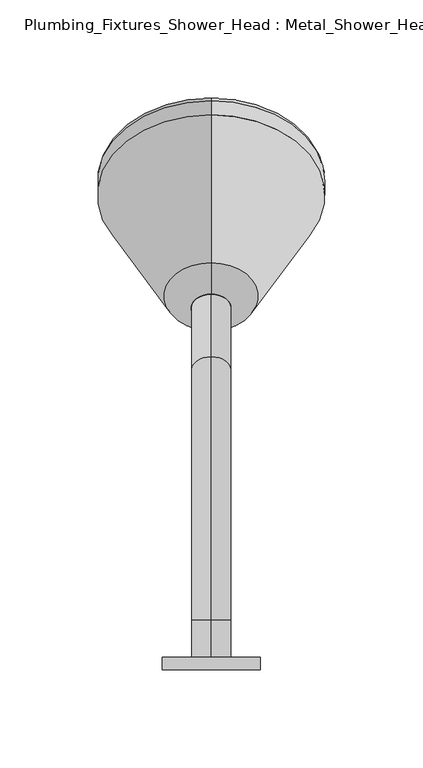
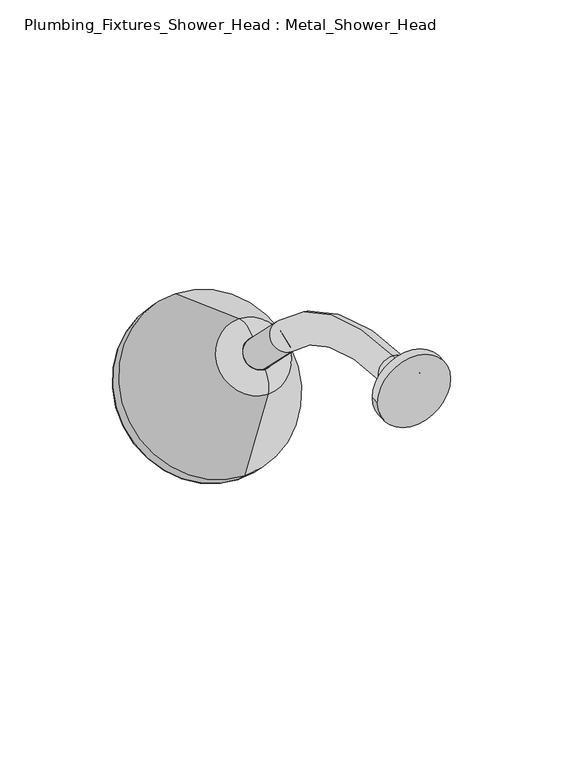
"""IFC4 building model written with IfcOpenShell, lengths in millimetres: flow terminal geometry, Plumbing_Fixtures_Shower_Head : Metal_Shower_Head."""

from ifc_helpers import new_model, si_unit, point, frame, frame_2d, origin, place, context, project, spatial, polyline, circle_curve, ellipse_curve, trimmed, segment, composite_curve, outline, extrude, source, transform, mapped, element, save
from ifc_brep_helpers import plane_surface, cylinder_surface, revolved_surface, advanced_brep


def plumbing_fixtures_shower_head_metal_shower_head_9404fff0(model_context):
    return source(origin(), model_context, "Body", "SolidModel", [
        advanced_brep(
        [(0.0, 6.4821489, 1590.0), (0.0, 6.4821489, 1610.0), (0.0, 25.4415588, 1590.0), (0.0, 25.4415588, 1610.0), (0.0, 159.7918472, 1554.3502884), (0.0, 145.6497116, 1540.2081528), (0.0, 177.4695167, 1508.3883476), (0.0, 191.6116524, 1522.5304833)],
        [
            (0, 1, circle_curve(frame((0.0, 6.4821489, 1600.0), z_axis=(0.0, -1.0, 0.0), x_axis=(0.0, 0.0, 1.0)), 10.0)),
            (1, 0, circle_curve(frame((0.0, 6.4821489, 1600.0), z_axis=(0.0, -1.0, 0.0), x_axis=(0.0, 0.0, 1.0)), 10.0)),
            (0, 2),
            (2, 3, circle_curve(frame((0.0, 25.4415588, 1600.0), z_axis=(0.0, -1.0, 0.0), x_axis=(0.0, 0.0, 1.0)), 10.0)),
            (3, 1),
            (3, 2, circle_curve(frame((0.0, 25.4415588, 1600.0), z_axis=(0.0, -1.0, 0.0), x_axis=(0.0, 0.0, 1.0)), 10.0)),
            (4, 3, circle_curve(frame((0.0, 25.4415588, 1420.0), z_axis=(1.0, 0.0, 0.0), x_axis=(0.0, 0.0, 1.0)), 190.0)),
            (2, 5, circle_curve(frame((0.0, 25.4415588, 1420.0), z_axis=(-1.0, 0.0, 0.0), x_axis=(0.0, 0.0, 1.0)), 170.0)),
            (5, 4, circle_curve(frame((0.0, 152.7207794, 1547.2792206), z_axis=(0.0, -0.7071067811865417, 0.7071067811865533), x_axis=(0.0, 0.7071067811865533, 0.7071067811865417)), 10.0)),
            (4, 5, circle_curve(frame((0.0, 152.7207794, 1547.2792206), z_axis=(0.0, -0.7071067811865416, 0.7071067811865535), x_axis=(0.0, 0.7071067811865535, 0.7071067811865416)), 10.0)),
            (6, 7, circle_curve(frame((0.0, 184.5405845, 1515.4594155), z_axis=(0.0, 0.7071067811865412, -0.7071067811865539), x_axis=(0.0, 0.7071067811865539, 0.7071067811865412)), 10.0)),
            (7, 6, circle_curve(frame((0.0, 184.5405845, 1515.4594155), z_axis=(0.0, 0.7071067811865412, -0.7071067811865539), x_axis=(0.0, 0.7071067811865539, 0.7071067811865412)), 10.0)),
            (5, 6),
            (7, 4),
        ],
        [
            plane_surface(frame((0.0, 6.4821489, 1600.0), z_axis=(0.0, -1.0, 0.0), x_axis=(1.0, 0.0, 0.0))),
            cylinder_surface(frame((0.0, 6.4821489, 1600.0), z_axis=(0.0, -1.0, 0.0), x_axis=(0.0, 0.0, 1.0)), 10.0),
            revolved_surface(trimmed(ellipse_curve(frame((0.0, 25.4415588, 1600.0), z_axis=(0.0, -1.0, 0.0), x_axis=(0.0, 0.0, 1.0)), 10.0, 10.0), [point((0.0, 25.4415588, 1590.0))], [point((0.0, 25.4415588, 1610.0))], True, "CARTESIAN"), (0.0, 25.4415588, 1420.0), (-1.0, 0.0, 0.0)),
            revolved_surface(trimmed(ellipse_curve(frame((0.0, 25.4415588, 1600.0), z_axis=(0.0, -1.0, 0.0), x_axis=(0.0, 0.0, 1.0)), 10.0, 10.0), [point((0.0, 25.4415588, 1610.0))], [point((0.0, 25.4415588, 1590.0))], True, "CARTESIAN"), (0.0, 25.4415588, 1420.0), (-1.0, 0.0, 0.0)),
            plane_surface(frame((0.0, 184.5405845, 1515.4594155), z_axis=(0.0, 0.7071067811865412, -0.7071067811865539), x_axis=(1.0, 0.0, 0.0))),
            cylinder_surface(frame((0.0, 152.7207794, 1547.2792206), z_axis=(0.0, -0.7071067811865412, 0.7071067811865539), x_axis=(0.0, 0.7071067811865539, 0.7071067811865412)), 10.0),
        ],
        [
            (0, [[1, 2]]),
            (1, [[-1, 3, 4, 5]]),
            (1, [[-2, -5, 6, -3]]),
            (2, [[7, -4, 8, 9]]),
            (3, [[-8, -6, -7, 10]]),
            (4, [[11, 12]]),
            (5, [[-9, 13, -12, 14]]),
            (5, [[-10, -14, -11, -13]]),
        ],
    ),
        advanced_brep(
        [(0.0, 207.6624735, 1526.3331882), (0.0, 173.6668118, 1492.3375265), (0.0, 177.1555994, 1508.0744304), (0.0, 191.9255696, 1522.8444006), (0.0, 283.255056, 1498.8197382), (0.0, 201.1802618, 1416.744944), (0.0, 290.3261238, 1491.7486704), (0.0, 208.2513296, 1409.6738762), (0.0, 290.3261238, 1484.6776026), (0.0, 215.3223974, 1409.6738762), (0.0, 288.6229509, 1482.9744296), (0.0, 217.0255704, 1411.3770491), (0.0, 287.2087373, 1484.3886432), (0.0, 215.6113568, 1412.7912627), (0.0, 251.4100471, 1448.5899529), (0.0, 184.5405845, 1515.4594155)],
        [
            (0, 1, circle_curve(frame((0.0, 190.6646427, 1509.3353573), z_axis=(0.0, -0.7071067811865374, 0.7071067811865579), x_axis=(0.0, -0.7071067811865579, -0.7071067811865374)), 24.0385629)),
            (1, 2, circle_curve(frame((0.0, 187.7622012, 1497.4678286), z_axis=(-1.0000000000000002, 0.0, 0.0), x_axis=(0.0, 1.0000000000000002, 0.0)), 15.0)),
            (2, 3, circle_curve(frame((0.0, 184.5405845, 1515.4594155), z_axis=(0.0, 0.7071067811865374, -0.7071067811865579), x_axis=(0.0, -0.7071067811865579, -0.7071067811865374)), 10.4439461)),
            (3, 0, circle_curve(frame((0.0, 202.5321714, 1512.2377988), z_axis=(-1.0000000000000002, 0.0, 0.0), x_axis=(0.0, 0.0, -1.0000000000000002)), 15.0)),
            (1, 0, circle_curve(frame((0.0, 190.6646427, 1509.3353573), z_axis=(0.0, -0.7071067811865374, 0.7071067811865579), x_axis=(0.0, -0.7071067811865579, -0.7071067811865374)), 24.0385629)),
            (3, 2, circle_curve(frame((0.0, 184.5405845, 1515.4594155), z_axis=(0.0, 0.7071067811865374, -0.7071067811865579), x_axis=(0.0, -0.7071067811865579, -0.7071067811865374)), 10.4439461)),
            (4, 5, circle_curve(frame((0.0, 242.2176589, 1457.7823411), z_axis=(0.0, -0.7071067811865374, 0.7071067811865579), x_axis=(0.0, -0.7071067811865579, -0.7071067811865374)), 58.0356436)),
            (5, 1),
            (0, 4),
            (5, 4, circle_curve(frame((0.0, 242.2176589, 1457.7823411), z_axis=(0.0, -0.7071067811865374, 0.7071067811865579), x_axis=(0.0, -0.7071067811865579, -0.7071067811865374)), 58.0356436)),
            (6, 7, circle_curve(frame((0.0, 249.2887267, 1450.7112733), z_axis=(0.0, -0.7071067811865374, 0.7071067811865579), x_axis=(0.0, -0.7071067811865579, -0.7071067811865374)), 58.0356436)),
            (7, 5),
            (4, 6),
            (7, 6, circle_curve(frame((0.0, 249.2887267, 1450.7112733), z_axis=(0.0, -0.7071067811865374, 0.7071067811865579), x_axis=(0.0, -0.7071067811865579, -0.7071067811865374)), 58.0356436)),
            (8, 9, circle_curve(frame((0.0, 252.8242606, 1447.1757394), z_axis=(0.0, -0.7071067811865374, 0.7071067811865579), x_axis=(0.0, -0.7071067811865579, -0.7071067811865374)), 53.0356436)),
            (9, 7, circle_curve(frame((0.0, 211.7868635, 1413.2094101), z_axis=(-1.0000000000000002, 0.0, 0.0), x_axis=(0.0, 1.0000000000000002, 0.0)), 5.0)),
            (6, 8, circle_curve(frame((0.0, 286.7905899, 1488.2131365), z_axis=(-1.0000000000000002, 0.0, 0.0), x_axis=(0.0, 0.0, -1.0000000000000002)), 5.0)),
            (9, 8, circle_curve(frame((0.0, 252.8242606, 1447.1757394), z_axis=(0.0, -0.7071067811865374, 0.7071067811865579), x_axis=(0.0, -0.7071067811865579, -0.7071067811865374)), 53.0356436)),
            (10, 11, circle_curve(frame((0.0, 252.8242606, 1447.1757394), z_axis=(0.0, -0.7071067811865374, 0.7071067811865579), x_axis=(0.0, -0.7071067811865579, -0.7071067811865374)), 50.6269933)),
            (11, 9),
            (8, 10),
            (11, 10, circle_curve(frame((0.0, 252.8242606, 1447.1757394), z_axis=(0.0, -0.7071067811865374, 0.7071067811865579), x_axis=(0.0, -0.7071067811865579, -0.7071067811865374)), 50.6269933)),
            (12, 13, circle_curve(frame((0.0, 251.4100471, 1448.5899529), z_axis=(0.0, -0.7071067811865374, 0.7071067811865579), x_axis=(0.0, -0.7071067811865579, -0.7071067811865374)), 50.6269933)),
            (13, 11),
            (10, 12),
            (13, 12, circle_curve(frame((0.0, 251.4100471, 1448.5899529), z_axis=(0.0, -0.7071067811865374, 0.7071067811865579), x_axis=(0.0, -0.7071067811865579, -0.7071067811865374)), 50.6269933)),
            (14, 13),
            (12, 14),
            (2, 15),
            (15, 3),
        ],
        [
            revolved_surface(trimmed(ellipse_curve(frame((0.0, 187.7622012, 1497.4678286), z_axis=(1.0000000000000002, 0.0, 0.0), x_axis=(0.0, 1.0000000000000002, 0.0)), 15.0, 15.0), [point((0.0, 177.1555994, 1508.0744304))], [point((0.0, 173.6668118, 1492.3375265))], True, "CARTESIAN"), (0.0, 184.5405845, 1515.4594155), (0.0, 0.7071067811865374, -0.7071067811865579)),
            revolved_surface(polyline([(0.0, 173.6668118, 1492.3375265), (0.0, 201.1802618, 1416.744944)]), (0.0, 184.5405845, 1515.4594155), (0.0, 0.7071067811865374, -0.7071067811865579)),
            cylinder_surface(frame((0.0, 184.5405845, 1515.4594155), z_axis=(0.0, 0.7071067811865374, -0.7071067811865579), x_axis=(0.0, -0.7071067811865579, -0.7071067811865374)), 58.0356436),
            revolved_surface(trimmed(ellipse_curve(frame((0.0, 211.7868635, 1413.2094101), z_axis=(1.0000000000000002, 0.0, 0.0), x_axis=(0.0, 1.0000000000000002, 0.0)), 5.0, 5.0), [point((0.0, 208.2513296, 1409.6738762))], [point((0.0, 215.3223974, 1409.6738762))], True, "CARTESIAN"), (0.0, 184.5405845, 1515.4594155), (0.0, 0.7071067811865374, -0.7071067811865579)),
            plane_surface(frame((0.0, 252.8242606, 1447.1757394), z_axis=(0.0, 0.7071067811865374, -0.7071067811865579), x_axis=(0.0, -0.7071067811865579, -0.7071067811865374))),
            revolved_surface(polyline([(0.0, 217.02557037648307, 1411.3770490764832), (0.0, 215.61135677648213, 1412.7912626764842)]), (0.0, 184.5405845, 1515.4594155), (0.0, 0.7071067811865374, -0.7071067811865579)),
            plane_surface(frame((0.0, 251.4100471, 1448.5899529), z_axis=(0.0, 0.7071067811865374, -0.7071067811865579), x_axis=(0.0, -0.7071067811865579, -0.7071067811865374))),
            plane_surface(frame((0.0, 184.5405845, 1515.4594155), z_axis=(0.0, -0.7071067811865374, 0.7071067811865579), x_axis=(0.0, -0.7071067811865579, -0.7071067811865374))),
        ],
        [
            (0, [[1, 2, 3, 4]]),
            (0, [[5, -4, 6, -2]]),
            (1, [[7, 8, -1, 9]]),
            (1, [[10, -9, -5, -8]]),
            (2, [[11, 12, -7, 13]]),
            (2, [[14, -13, -10, -12]]),
            (3, [[15, 16, -11, 17]]),
            (3, [[18, -17, -14, -16]]),
            (4, [[19, 20, -15, 21]]),
            (4, [[22, -21, -18, -20]]),
            (5, [[23, 24, -19, 25]]),
            (5, [[26, -25, -22, -24]]),
            (6, [[27, -23, 28]]),
            (6, [[-28, -26, -27]]),
            (7, [[-3, 29, 30]]),
            (7, [[-6, -30, -29]]),
        ],
    ),
        extrude(outline(composite_curve([segment(trimmed(circle_curve(frame_2d((1600.0, 0.0)), 25.0), [point((1600.0, -25.0))], [point((1600.0, 25.0))], False, "CARTESIAN"), True, "CONTINUOUS"), segment(trimmed(circle_curve(frame_2d((1600.0, 0.0)), 25.0), [point((1600.0, 25.0))], [point((1600.0, -25.0))], False, "CARTESIAN"), True, "CONTINUOUS")], self_intersect=False)), frame((0.0, 0.0, 0.0), z_axis=(0.0, 1.0, 0.0), x_axis=(0.0, 0.0, 1.0)), (0.0, 0.0, 1.0), 6.4821489),
    ])


if __name__ == "__main__":
    model = new_model("IFC4")
    model_context = context("Model", 3, world=origin())
    ifc_project = project(units=[si_unit("LENGTHUNIT", "METRE", prefix="MILLI")], contexts=[model_context])
    site = spatial("IfcSite", under=ifc_project)
    building = spatial("IfcBuilding", under=site)
    placement = place(None, origin())
    plumbing_fixtures_shower_head_metal_shower_head_shape = plumbing_fixtures_shower_head_metal_shower_head_9404fff0(model_context)
    element("IfcFlowTerminal", 1, ObjectType="Plumbing_Fixtures_Shower_Head : Metal_Shower_Head", at=placement, inside=building, context=model_context, shape_type="MappedRepresentation", body=[
        mapped(plumbing_fixtures_shower_head_metal_shower_head_shape, transform((0.0, 0.0, 0.0), x_axis=(1.0, 0.0, 0.0), y_axis=(0.0, 1.0, 0.0), z_axis=(0.0, 0.0, 1.0))),
    ])
    save(model, "model.ifc")

# Revit data of these elements
# Type "Plumbing_Fixtures_Shower_Head : Metal_Shower_Head"
#   Keynote = "N13/230"
#   Mounting Height = 1600 mm
#   Material Shower Head = Metal - Chrome Polished
#   Default Elevation = 0
# Element 1 (IfcFlowTerminal, "Plumbing_Fixtures_Shower_Head : Metal_Shower_Head")
#   Materials on its faces: "Metal - Chrome Polished"
# Materials
#   "Metal - Chrome Polished": colour RGB 247 247 247, transparency 0
